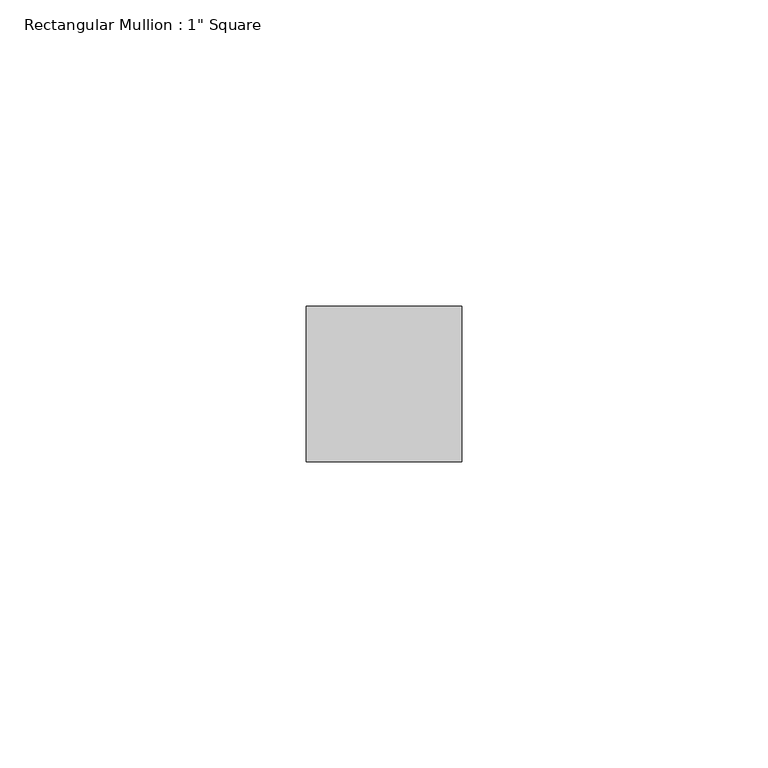
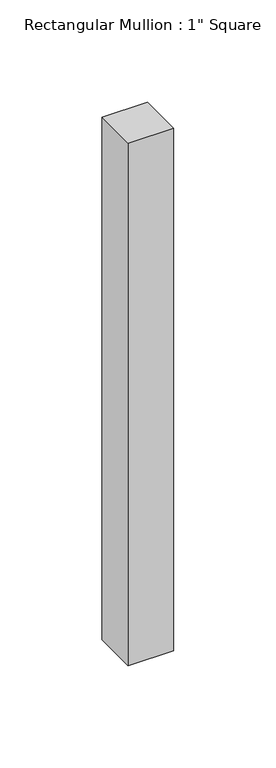
"""IFC4 building model written with IfcOpenShell, lengths in millimetres: member geometry."""

from ifc_helpers import new_model, si_unit, frame, origin, place, context, project, spatial, polyline, outline, extrude, source, transform, mapped, element, save


def member_2c71ef08(model_context):
    return source(origin(), model_context, "Body", "SweptSolid", [
        extrude(outline(polyline([(12.7, 12.7), (12.7, -12.7), (-12.7, -12.7), (-12.7, 12.7), (12.7, 12.7)])), frame((0.0, 0.0, -311.15), z_axis=(0.0, 0.0, 1.0), x_axis=(1.0, 0.0, 0.0)), (0.0, 0.0, 1.0), 311.15),
    ])


if __name__ == "__main__":
    model = new_model("IFC4")
    model_context = context("Model", 3, world=origin())
    ifc_project = project(units=[si_unit("LENGTHUNIT", "METRE", prefix="MILLI")], contexts=[model_context])
    site = spatial("IfcSite", under=ifc_project)
    building = spatial("IfcBuilding", under=site)
    placement = place(None, origin())
    member_shape = member_2c71ef08(model_context)
    element("IfcMember", 1, ObjectType="Rectangular Mullion : 1\" Square", at=placement, inside=building, context=model_context, shape_type="MappedRepresentation", body=[
        mapped(member_shape, transform((0.0, 0.0, 0.0), x_axis=(1.0, 0.0, 0.0), y_axis=(0.0, 1.0, 0.0), z_axis=(0.0, 0.0, 1.0))),
    ])
    save(model, "model.ifc")

# Revit data of these elements
# Type "Rectangular Mullion : 1\" Square"
#   built-in parameter 1007304 = 0.0833333 (stored number, unit not read)
#   built-in parameter 1007301 = 0.0416667 (stored number, unit not read)
#   built-in parameter 1007300 = 0.0416667 (stored number, unit not read)
